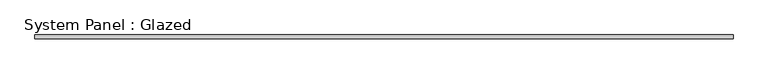
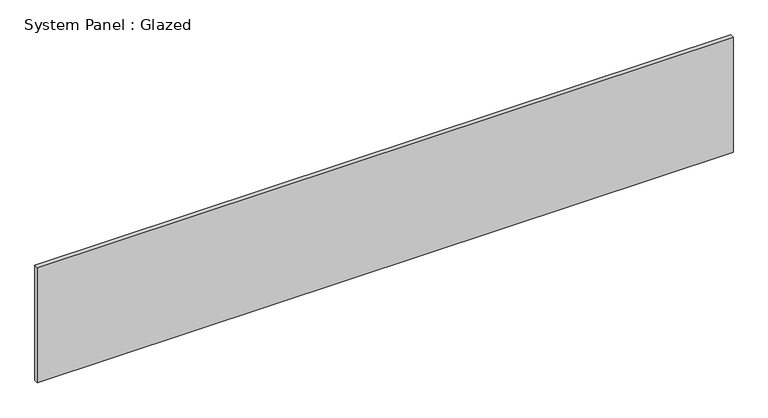
"""IFC4 building model written with IfcOpenShell, lengths in millimetres: plate geometry, System Panel : Glazed."""

from ifc_helpers import new_model, si_unit, origin, origin_with_axes, place, context, project, spatial, polyline, outline, extrude, source, transform, mapped, element, save


def system_panel_glazed_4996dcf2(model_context):
    return source(origin(), model_context, "Body", "SweptSolid", [
        extrude(outline(polyline([(2260.6, 19.05), (-2260.6, 19.05), (-2260.6, 44.45), (2260.6, 44.45), (2260.6, 19.05)])), origin_with_axes(), (0.0, 0.0, 1.0), 790.1180586),
    ])


if __name__ == "__main__":
    model = new_model("IFC4")
    model_context = context("Model", 3, world=origin())
    ifc_project = project(units=[si_unit("LENGTHUNIT", "METRE", prefix="MILLI")], contexts=[model_context])
    site = spatial("IfcSite", under=ifc_project)
    building = spatial("IfcBuilding", under=site)
    placement = place(None, origin())
    system_panel_glazed_shape = system_panel_glazed_4996dcf2(model_context)
    element("IfcPlate", 1, ObjectType="System Panel : Glazed", at=placement, inside=building, context=model_context, shape_type="MappedRepresentation", body=[
        mapped(system_panel_glazed_shape, transform((0.0, 0.0, 0.0), x_axis=(1.0, 0.0, 0.0), y_axis=(0.0, 1.0, 0.0), z_axis=(0.0, 0.0, 1.0))),
    ])
    save(model, "model.ifc")

# Revit data of these elements
# Type "System Panel : Glazed"
#   Construction Type Id = "GSP4R"
#   Analytic Construction = "1/8 in Pilkington single glazing"
#   Visual Light Transmittance = 0.9
#   Solar Heat Gain Coefficient = 0.86
#   Heat Transfer Coefficient (U) = 1.18115 BTU/(h·ft²·°F)
#   Define Thermal Properties by = 1
# Element 1 (IfcPlate, "System Panel : Glazed")
#   Materials on its faces: "Glass"
# Materials
#   "Glass": class "Glass", colour RGB 0 128 192, transparency 0.75, Description = "Soda Lime Glass", Cost = 0
